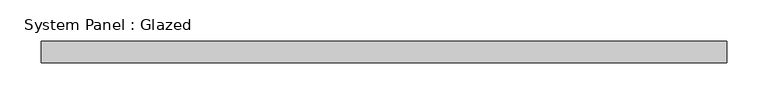
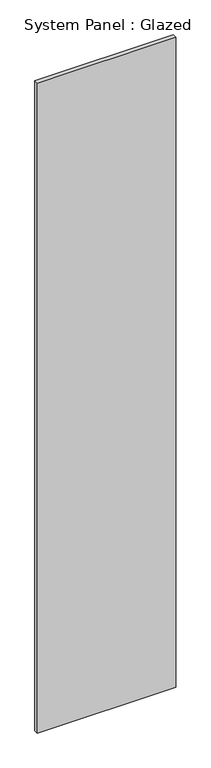
"""IFC4 building model written with IfcOpenShell, lengths in millimetres: plate geometry, System Panel : Glazed."""

from ifc_helpers import new_model, si_unit, origin, origin_with_axes, place, context, project, spatial, polyline, outline, extrude, source, transform, mapped, element, save


def system_panel_glazed_14c0cd2a(model_context):
    return source(origin(), model_context, "Body", "SweptSolid", [
        extrude(outline(polyline([(412.75, 19.05), (-412.75, 19.05), (-412.75, 44.45), (412.75, 44.45), (412.75, 19.05)])), origin_with_axes(), (0.0, 0.0, 1.0), 4103.04239),
    ])


if __name__ == "__main__":
    model = new_model("IFC4")
    model_context = context("Model", 3, world=origin())
    ifc_project = project(units=[si_unit("LENGTHUNIT", "METRE", prefix="MILLI")], contexts=[model_context])
    site = spatial("IfcSite", under=ifc_project)
    building = spatial("IfcBuilding", under=site)
    placement = place(None, origin())
    system_panel_glazed_shape = system_panel_glazed_14c0cd2a(model_context)
    element("IfcPlate", 1, ObjectType="System Panel : Glazed", at=placement, inside=building, context=model_context, shape_type="MappedRepresentation", body=[
        mapped(system_panel_glazed_shape, transform((0.0, 0.0, 0.0), x_axis=(1.0, 0.0, 0.0), y_axis=(0.0, 1.0, 0.0), z_axis=(0.0, 0.0, 1.0))),
    ])
    save(model, "model.ifc")

# Revit data of these elements
# Type "System Panel : Glazed"
#   Construction Type Id = "GSP4R"
#   Analytic Construction = "1/8 in Pilkington single glazing"
#   Visual Light Transmittance = 0.9
#   Solar Heat Gain Coefficient = 0.86
#   Heat Transfer Coefficient (U) = 1.18115 BTU/(h·ft²·°F)
#   Define Thermal Properties by = 1
# Element 1 (IfcPlate, "System Panel : Glazed")
#   Materials on its faces: "Glass"
# Materials
#   "Glass": class "Glass", colour RGB 0 128 192, transparency 0.75, Description = "Soda Lime Glass", Cost = 0
